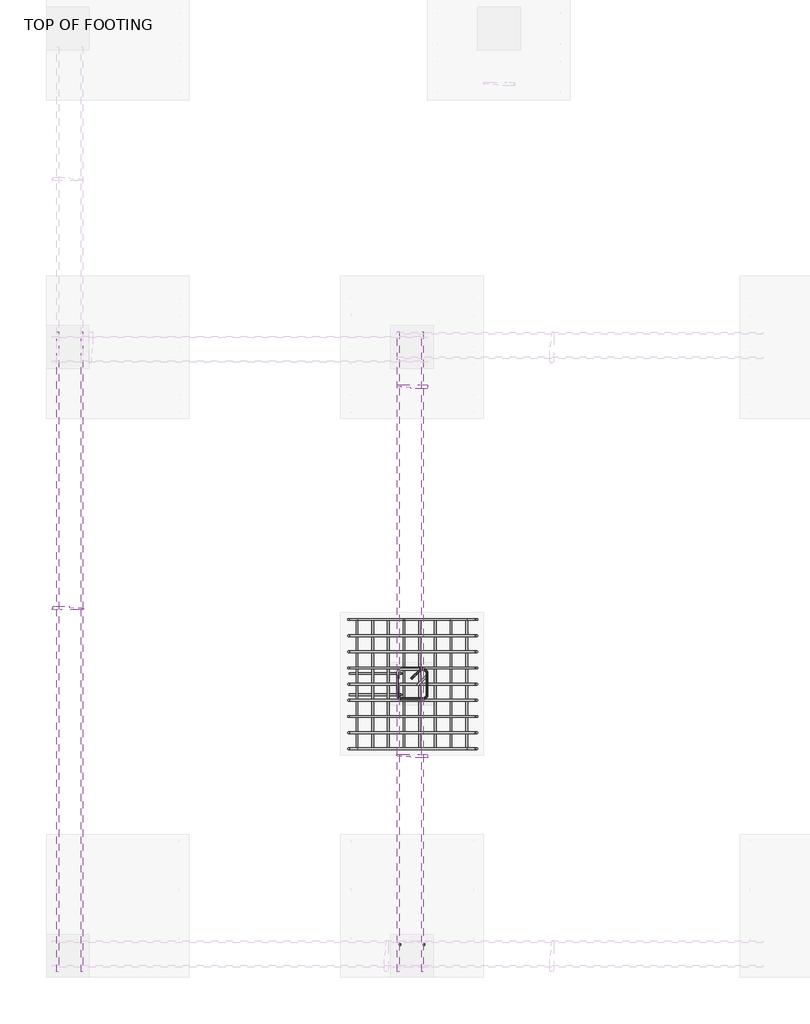
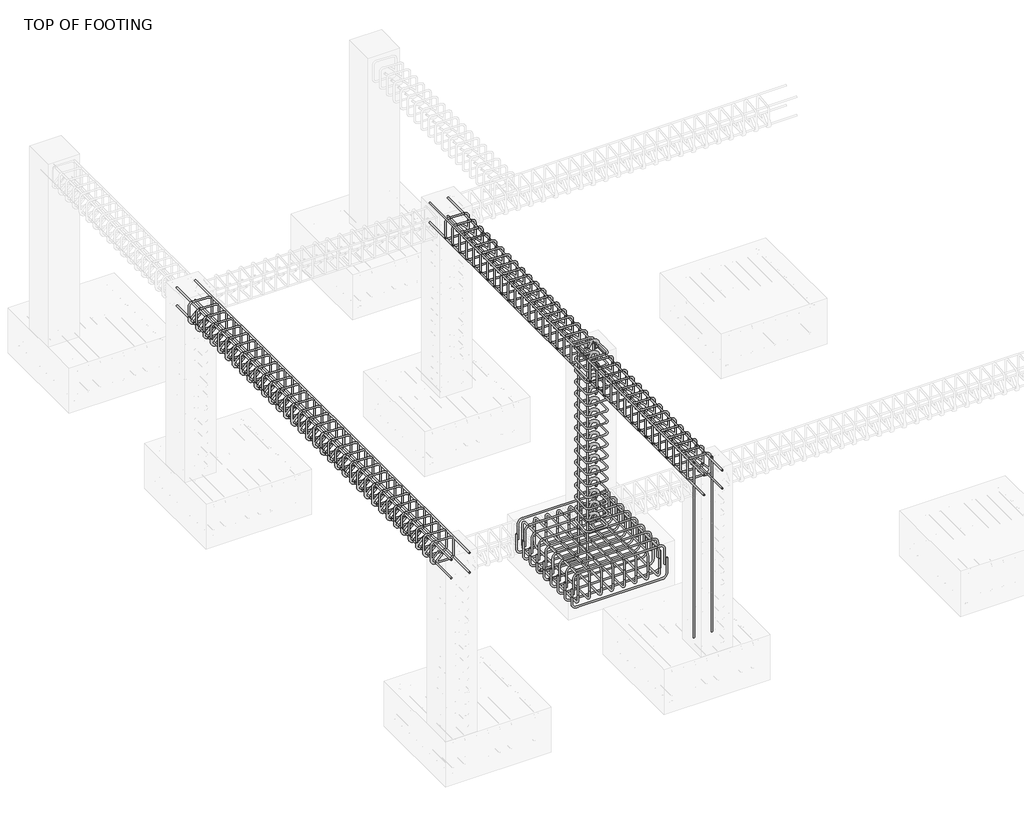
# One storey, part 3 of 10: 16 reinforcing bars.
"""IFC4 building model written with IfcOpenShell, lengths in millimetres."""

from ifc_helpers import new_model, si_unit, point, frame, origin, place, context, project, spatial, polyline, circle_curve, trimmed, segment, composite_curve, source, transform, mapped, element, save
from ifc_brep_helpers import swept_disk

model = new_model("IFC4")

# Units and contexts
model_context = context("Model", 3, world=origin())
ifc_project = project(units=[si_unit("LENGTHUNIT", "METRE", prefix="MILLI")], contexts=[model_context])

# Site, building, storey
site = spatial("IfcSite", under=ifc_project)
building = spatial("IfcBuilding", under=site)
storey = spatial("IfcBuildingStorey", under=building, Name="TOP OF FOOTING", Elevation=-1828.8)

# Reinforcing bars
placement = place(None, origin())
reinforcing_bar_shape = source(origin(), model_context, "Body", "SolidModel", [
    swept_disk(composite_curve([segment(polyline([(-7671.9957678, 10418.4767485, -2013.6880036), (-7671.9957678, 10418.4767485, -2160.9880036)]), True, "CONTINUOUS"), segment(trimmed(circle_curve(frame((-7718.3457678, 10418.4767485, -2160.9880036), z_axis=(0.0, 1.0, 0.0), x_axis=(46.350000000000364, 0.0, 0.0)), 46.35), [point((-7671.9957678, 10418.4767485, -2160.9880036))], [point((-7718.3457678, 10418.4767485, -2207.3380036))], True, "CARTESIAN"), True, "CONTINUOUS"), segment(polyline([(-7718.3457678, 10418.4767485, -2207.3380036), (-8526.0530437, 10418.4767485, -2207.3380036)]), True, "CONTINUOUS"), segment(trimmed(circle_curve(frame((-8526.0530437, 10418.4767485, -2160.9880036), z_axis=(0.0, 1.0, 0.0), x_axis=(0.0, 0.0, -46.34999999999991)), 46.35), [point((-8526.0530437, 10418.4767485, -2207.3380036))], [point((-8572.4030437, 10418.4767485, -2160.9880036))], True, "CARTESIAN"), True, "CONTINUOUS"), segment(polyline([(-8572.4030437, 10418.4767485, -2160.9880036), (-8572.4030437, 10418.4767485, -2013.6880036)]), True, "CONTINUOUS")], self_intersect=False), 6.35),
])
element("IfcReinforcingBar", 1, at=placement, inside=storey, context=model_context, shape_type="MappedRepresentation", body=[
    mapped(reinforcing_bar_shape, transform((0.0, 0.0, 0.0), x_axis=(1.0, 0.0, 0.0), y_axis=(0.0, 1.0, 0.0), z_axis=(0.0, 0.0, 1.0))),
    mapped(reinforcing_bar_shape, transform((0.0, -113.4125, 0.0), x_axis=(1.0, 0.0, 0.0), y_axis=(0.0, 1.0, 0.0), z_axis=(0.0, 0.0, 1.0))),
    mapped(reinforcing_bar_shape, transform((0.0, -226.825, 0.0), x_axis=(1.0, 0.0, 0.0), y_axis=(0.0, 1.0, 0.0), z_axis=(0.0, 0.0, 1.0))),
    mapped(reinforcing_bar_shape, transform((0.0, -340.2375, 0.0), x_axis=(1.0, 0.0, 0.0), y_axis=(0.0, 1.0, 0.0), z_axis=(0.0, 0.0, 1.0))),
    mapped(reinforcing_bar_shape, transform((0.0, -453.65, 0.0), x_axis=(1.0, 0.0, 0.0), y_axis=(0.0, 1.0, 0.0), z_axis=(0.0, 0.0, 1.0))),
    mapped(reinforcing_bar_shape, transform((0.0, -567.0625, 0.0), x_axis=(1.0, 0.0, 0.0), y_axis=(0.0, 1.0, 0.0), z_axis=(0.0, 0.0, 1.0))),
    mapped(reinforcing_bar_shape, transform((0.0, -680.475, 0.0), x_axis=(1.0, 0.0, 0.0), y_axis=(0.0, 1.0, 0.0), z_axis=(0.0, 0.0, 1.0))),
    mapped(reinforcing_bar_shape, transform((0.0, -793.8875, 0.0), x_axis=(1.0, 0.0, 0.0), y_axis=(0.0, 1.0, 0.0), z_axis=(0.0, 0.0, 1.0))),
    mapped(reinforcing_bar_shape, transform((0.0, -907.3, 0.0), x_axis=(1.0, 0.0, 0.0), y_axis=(0.0, 1.0, 0.0), z_axis=(0.0, 0.0, 1.0))),
])
reinforcing_bar_2_shape = source(origin(), model_context, "Body", "SolidModel", [
    swept_disk(composite_curve([segment(polyline([(-8556.1548549, 10418.4767485, -2068.7560969), (-8556.1548549, 10418.4767485, -1921.4560969)]), True, "CONTINUOUS"), segment(trimmed(circle_curve(frame((-8509.8048549, 10418.4767485, -1921.4560969), z_axis=(0.0, 1.0, 0.0), x_axis=(-46.350000000000364, 0.0, 0.0)), 46.35), [point((-8556.1548549, 10418.4767485, -1921.4560969))], [point((-8509.8048549, 10418.4767485, -1875.1060969))], True, "CARTESIAN"), True, "CONTINUOUS"), segment(polyline([(-8509.8048549, 10418.4767485, -1875.1060969), (-7741.4133686, 10418.4767485, -1875.1060969)]), True, "CONTINUOUS"), segment(trimmed(circle_curve(frame((-7741.4133686, 10418.4767485, -1921.4560969), z_axis=(0.0, 1.0, 0.0), x_axis=(0.0, 0.0, 46.34999999999991)), 46.35), [point((-7741.4133686, 10418.4767485, -1875.1060969))], [point((-7695.0633686, 10418.4767485, -1921.4560969))], True, "CARTESIAN"), True, "CONTINUOUS"), segment(polyline([(-7695.0633686, 10418.4767485, -1921.4560969), (-7695.0633686, 10418.4767485, -2068.7560969)]), True, "CONTINUOUS")], self_intersect=False), 6.35),
])
element("IfcReinforcingBar", 2, at=placement, inside=storey, context=model_context, shape_type="MappedRepresentation", body=[
    mapped(reinforcing_bar_2_shape, transform((0.0, 0.0, 0.0), x_axis=(1.0, 0.0, 0.0), y_axis=(0.0, 1.0, 0.0), z_axis=(0.0, 0.0, 1.0))),
    mapped(reinforcing_bar_2_shape, transform((0.0, -113.4125, 0.0), x_axis=(1.0, 0.0, 0.0), y_axis=(0.0, 1.0, 0.0), z_axis=(0.0, 0.0, 1.0))),
    mapped(reinforcing_bar_2_shape, transform((0.0, -226.825, 0.0), x_axis=(1.0, 0.0, 0.0), y_axis=(0.0, 1.0, 0.0), z_axis=(0.0, 0.0, 1.0))),
    mapped(reinforcing_bar_2_shape, transform((0.0, -340.2375, 0.0), x_axis=(1.0, 0.0, 0.0), y_axis=(0.0, 1.0, 0.0), z_axis=(0.0, 0.0, 1.0))),
    mapped(reinforcing_bar_2_shape, transform((0.0, -453.65, 0.0), x_axis=(1.0, 0.0, 0.0), y_axis=(0.0, 1.0, 0.0), z_axis=(0.0, 0.0, 1.0))),
    mapped(reinforcing_bar_2_shape, transform((0.0, -567.0625, 0.0), x_axis=(1.0, 0.0, 0.0), y_axis=(0.0, 1.0, 0.0), z_axis=(0.0, 0.0, 1.0))),
    mapped(reinforcing_bar_2_shape, transform((0.0, -680.475, 0.0), x_axis=(1.0, 0.0, 0.0), y_axis=(0.0, 1.0, 0.0), z_axis=(0.0, 0.0, 1.0))),
    mapped(reinforcing_bar_2_shape, transform((0.0, -793.8875, 0.0), x_axis=(1.0, 0.0, 0.0), y_axis=(0.0, 1.0, 0.0), z_axis=(0.0, 0.0, 1.0))),
    mapped(reinforcing_bar_2_shape, transform((0.0, -907.3, 0.0), x_axis=(1.0, 0.0, 0.0), y_axis=(0.0, 1.0, 0.0), z_axis=(0.0, 0.0, 1.0))),
])
reinforcing_bar_3_shape = source(origin(), model_context, "Body", "SolidModel", [
    swept_disk(composite_curve([segment(polyline([(-7744.2682872, 10418.4767485, -2087.4821199), (-7744.2682872, 10418.4767485, -1940.1821199)]), True, "CONTINUOUS"), segment(trimmed(circle_curve(frame((-7744.2682872, 10372.1267485, -1940.1821199), z_axis=(1.0, 0.0, 0.0), x_axis=(0.0, 46.349999999998545, 0.0)), 46.35), [point((-7744.2682872, 10418.4767485, -1940.1821199))], [point((-7744.2682872, 10372.1267485, -1893.8321199))], True, "CARTESIAN"), True, "CONTINUOUS"), segment(polyline([(-7744.2682872, 10372.1267485, -1893.8321199), (-7744.2682872, 9557.5267485, -1893.8321199)]), True, "CONTINUOUS"), segment(trimmed(circle_curve(frame((-7744.2682872, 9557.5267485, -1940.1821199), z_axis=(1.0, 0.0, 0.0), x_axis=(0.0, 0.0, 46.350000000000136)), 46.35), [point((-7744.2682872, 9557.5267485, -1893.8321199))], [point((-7744.2682872, 9511.1767485, -1940.1821199))], True, "CARTESIAN"), True, "CONTINUOUS"), segment(polyline([(-7744.2682872, 9511.1767485, -1940.1821199), (-7744.2682872, 9511.1767485, -2087.4821199)]), True, "CONTINUOUS")], self_intersect=False), 6.35),
])
element("IfcReinforcingBar", 3, at=placement, inside=storey, context=model_context, shape_type="MappedRepresentation", body=[
    mapped(reinforcing_bar_3_shape, transform((0.0, 0.0, 0.0), x_axis=(1.0, 0.0, 0.0), y_axis=(0.0, 1.0, 0.0), z_axis=(0.0, 0.0, 1.0))),
    mapped(reinforcing_bar_3_shape, transform((-109.824938, 0.0, 0.0), x_axis=(1.0, 0.0, 0.0), y_axis=(0.0, 1.0, 0.0), z_axis=(0.0, 0.0, 1.0))),
    mapped(reinforcing_bar_3_shape, transform((-219.649876, 0.0, 0.0), x_axis=(1.0, 0.0, 0.0), y_axis=(0.0, 1.0, 0.0), z_axis=(0.0, 0.0, 1.0))),
    mapped(reinforcing_bar_3_shape, transform((-329.474814, 0.0, 0.0), x_axis=(1.0, 0.0, 0.0), y_axis=(0.0, 1.0, 0.0), z_axis=(0.0, 0.0, 1.0))),
    mapped(reinforcing_bar_3_shape, transform((-439.299752, 0.0, 0.0), x_axis=(1.0, 0.0, 0.0), y_axis=(0.0, 1.0, 0.0), z_axis=(0.0, 0.0, 1.0))),
    mapped(reinforcing_bar_3_shape, transform((-549.12469, 0.0, 0.0), x_axis=(1.0, 0.0, 0.0), y_axis=(0.0, 1.0, 0.0), z_axis=(0.0, 0.0, 1.0))),
    mapped(reinforcing_bar_3_shape, transform((-658.949628, 0.0, 0.0), x_axis=(1.0, 0.0, 0.0), y_axis=(0.0, 1.0, 0.0), z_axis=(0.0, 0.0, 1.0))),
    mapped(reinforcing_bar_3_shape, transform((-768.774566, 0.0, 0.0), x_axis=(1.0, 0.0, 0.0), y_axis=(0.0, 1.0, 0.0), z_axis=(0.0, 0.0, 1.0))),
])
reinforcing_bar_4_shape = source(origin(), model_context, "Body", "SolidModel", [
    swept_disk(composite_curve([segment(polyline([(-8513.0428532, 10418.4767485, -1990.1985611), (-8513.0428532, 10418.4767485, -2137.4985611)]), True, "CONTINUOUS"), segment(trimmed(circle_curve(frame((-8513.0428532, 10372.1267485, -2137.4985611), z_axis=(-1.0, 0.0, 0.0), x_axis=(0.0, 46.349999999998545, 0.0)), 46.35), [point((-8513.0428532, 10418.4767485, -2137.4985611))], [point((-8513.0428532, 10372.1267485, -2183.8485611))], True, "CARTESIAN"), True, "CONTINUOUS"), segment(polyline([(-8513.0428532, 10372.1267485, -2183.8485611), (-8513.0428532, 9557.5267485, -2183.8485611)]), True, "CONTINUOUS"), segment(trimmed(circle_curve(frame((-8513.0428532, 9557.5267485, -2137.4985611), z_axis=(-1.0, 0.0, 0.0), x_axis=(0.0, 0.0, -46.34999999999991)), 46.35), [point((-8513.0428532, 9557.5267485, -2183.8485611))], [point((-8513.0428532, 9511.1767485, -2137.4985611))], True, "CARTESIAN"), True, "CONTINUOUS"), segment(polyline([(-8513.0428532, 9511.1767485, -2137.4985611), (-8513.0428532, 9511.1767485, -1990.1985611)]), True, "CONTINUOUS")], self_intersect=False), 6.35),
])
element("IfcReinforcingBar", 4, at=placement, inside=storey, context=model_context, shape_type="MappedRepresentation", body=[
    mapped(reinforcing_bar_4_shape, transform((0.0, 0.0, 0.0), x_axis=(1.0, 0.0, 0.0), y_axis=(0.0, 1.0, 0.0), z_axis=(0.0, 0.0, 1.0))),
    mapped(reinforcing_bar_4_shape, transform((109.824938, 0.0, 0.0), x_axis=(1.0, 0.0, 0.0), y_axis=(0.0, 1.0, 0.0), z_axis=(0.0, 0.0, 1.0))),
    mapped(reinforcing_bar_4_shape, transform((219.649876, 0.0, 0.0), x_axis=(1.0, 0.0, 0.0), y_axis=(0.0, 1.0, 0.0), z_axis=(0.0, 0.0, 1.0))),
    mapped(reinforcing_bar_4_shape, transform((329.474814, 0.0, 0.0), x_axis=(1.0, 0.0, 0.0), y_axis=(0.0, 1.0, 0.0), z_axis=(0.0, 0.0, 1.0))),
    mapped(reinforcing_bar_4_shape, transform((439.299752, 0.0, 0.0), x_axis=(1.0, 0.0, 0.0), y_axis=(0.0, 1.0, 0.0), z_axis=(0.0, 0.0, 1.0))),
    mapped(reinforcing_bar_4_shape, transform((549.12469, 0.0, 0.0), x_axis=(1.0, 0.0, 0.0), y_axis=(0.0, 1.0, 0.0), z_axis=(0.0, 0.0, 1.0))),
    mapped(reinforcing_bar_4_shape, transform((658.949628, 0.0, 0.0), x_axis=(1.0, 0.0, 0.0), y_axis=(0.0, 1.0, 0.0), z_axis=(0.0, 0.0, 1.0))),
    mapped(reinforcing_bar_4_shape, transform((768.774566, 0.0, 0.0), x_axis=(1.0, 0.0, 0.0), y_axis=(0.0, 1.0, 0.0), z_axis=(0.0, 0.0, 1.0))),
])
reinforcing_bar_5_shape = source(origin(), model_context, "Body", "SolidModel", [
    swept_disk(composite_curve([segment(polyline([(-8131.2571284, 10003.5509831, -57.3273613), (-8075.5135654, 10059.2945461, -57.3273613)]), True, "CONTINUOUS"), segment(trimmed(circle_curve(frame((-8053.3457678, 10037.1267485, -57.3273613), z_axis=(0.0, 0.0, -1.0), x_axis=(-22.167797599999176, 22.167797599999176, 0.0)), 31.35), [point((-8075.5135654, 10059.2945461, -57.3273613))], [point((-8021.9957678, 10037.1267485, -57.3273613))], True, "CARTESIAN"), True, "CONTINUOUS"), segment(polyline([(-8021.9957678, 10037.1267485, -57.3273613), (-8021.9957678, 9892.5267485, -57.3273613)]), True, "CONTINUOUS"), segment(trimmed(circle_curve(frame((-8053.3457678, 9892.5267485, -57.3273613), z_axis=(0.0, 0.0, -1.0), x_axis=(31.350000000000364, 0.0, 0.0)), 31.35), [point((-8021.9957678, 9892.5267485, -57.3273613))], [point((-8053.3457678, 9861.1767485, -57.3273613))], True, "CARTESIAN"), True, "CONTINUOUS"), segment(polyline([(-8053.3457678, 9861.1767485, -57.3273613), (-8197.9457678, 9861.1767485, -57.3273613)]), True, "CONTINUOUS"), segment(trimmed(circle_curve(frame((-8197.9457678, 9892.4680812, -55.4103332), z_axis=(0.0, 0.06114922175001322, -0.9981286353368326), x_axis=(0.0, -31.291332700000567, -1.9170281000000031)), 31.35), [point((-8197.9457678, 9861.1767485, -57.3273613))], [point((-8229.2957678, 9892.4680812, -55.4103332))], True, "CARTESIAN"), True, "CONTINUOUS"), segment(polyline([(-8229.2957678, 9892.4680812, -55.4103332), (-8229.2957678, 10037.1854158, -46.5443894)]), True, "CONTINUOUS"), segment(trimmed(circle_curve(frame((-8197.9457678, 10037.1854158, -46.5443894), z_axis=(0.0, 0.06114922175001322, -0.9981286353368326), x_axis=(-31.350000000000364, 0.0, 0.0)), 31.35), [point((-8229.2957678, 10037.1854158, -46.5443894))], [point((-8197.9457678, 10068.4767485, -44.6273613))], True, "CARTESIAN"), True, "CONTINUOUS"), segment(polyline([(-8197.9457678, 10068.4767485, -44.6273613), (-8053.3457678, 10068.4767485, -44.6273613)]), True, "CONTINUOUS"), segment(trimmed(circle_curve(frame((-8053.3457678, 10037.1267485, -44.6273613), z_axis=(0.0, 0.0, -1.0), x_axis=(0.0, 31.349999999998545, 0.0)), 31.35), [point((-8053.3457678, 10068.4767485, -44.6273613))], [point((-8031.1779702, 10014.9589509, -44.6273613))], True, "CARTESIAN"), True, "CONTINUOUS"), segment(polyline([(-8031.1779702, 10014.9589509, -44.6273613), (-8086.9215332, 9959.2153879, -44.6273613)]), True, "CONTINUOUS")], self_intersect=False), 6.35),
])
element("IfcReinforcingBar", 5, at=placement, inside=storey, context=model_context, shape_type="MappedRepresentation", body=[
    mapped(reinforcing_bar_5_shape, transform((0.0, 0.0, 0.0), x_axis=(1.0, 0.0, 0.0), y_axis=(0.0, 1.0, 0.0), z_axis=(0.0, 0.0, 1.0))),
    mapped(reinforcing_bar_5_shape, transform((0.0, 0.0, -115.0081759), x_axis=(1.0, 0.0, 0.0), y_axis=(0.0, 1.0, 0.0), z_axis=(0.0, 0.0, 1.0))),
    mapped(reinforcing_bar_5_shape, transform((0.0, 0.0, -230.0163518), x_axis=(1.0, 0.0, 0.0), y_axis=(0.0, 1.0, 0.0), z_axis=(0.0, 0.0, 1.0))),
    mapped(reinforcing_bar_5_shape, transform((0.0, 0.0, -345.0245277), x_axis=(1.0, 0.0, 0.0), y_axis=(0.0, 1.0, 0.0), z_axis=(0.0, 0.0, 1.0))),
    mapped(reinforcing_bar_5_shape, transform((0.0, 0.0, -460.0327037), x_axis=(1.0, 0.0, 0.0), y_axis=(0.0, 1.0, 0.0), z_axis=(0.0, 0.0, 1.0))),
    mapped(reinforcing_bar_5_shape, transform((0.0, 0.0, -575.0408796), x_axis=(1.0, 0.0, 0.0), y_axis=(0.0, 1.0, 0.0), z_axis=(0.0, 0.0, 1.0))),
    mapped(reinforcing_bar_5_shape, transform((0.0, 0.0, -690.0490555), x_axis=(1.0, 0.0, 0.0), y_axis=(0.0, 1.0, 0.0), z_axis=(0.0, 0.0, 1.0))),
    mapped(reinforcing_bar_5_shape, transform((0.0, 0.0, -805.0572314), x_axis=(1.0, 0.0, 0.0), y_axis=(0.0, 1.0, 0.0), z_axis=(0.0, 0.0, 1.0))),
    mapped(reinforcing_bar_5_shape, transform((0.0, 0.0, -920.0654073), x_axis=(1.0, 0.0, 0.0), y_axis=(0.0, 1.0, 0.0), z_axis=(0.0, 0.0, 1.0))),
    mapped(reinforcing_bar_5_shape, transform((0.0, 0.0, -1035.0735832), x_axis=(1.0, 0.0, 0.0), y_axis=(0.0, 1.0, 0.0), z_axis=(0.0, 0.0, 1.0))),
    mapped(reinforcing_bar_5_shape, transform((0.0, 0.0, -1150.0817591), x_axis=(1.0, 0.0, 0.0), y_axis=(0.0, 1.0, 0.0), z_axis=(0.0, 0.0, 1.0))),
    mapped(reinforcing_bar_5_shape, transform((0.0, 0.0, -1265.0899351), x_axis=(1.0, 0.0, 0.0), y_axis=(0.0, 1.0, 0.0), z_axis=(0.0, 0.0, 1.0))),
    mapped(reinforcing_bar_5_shape, transform((0.0, 0.0, -1380.098111), x_axis=(1.0, 0.0, 0.0), y_axis=(0.0, 1.0, 0.0), z_axis=(0.0, 0.0, 1.0))),
    mapped(reinforcing_bar_5_shape, transform((0.0, 0.0, -1495.1062869), x_axis=(1.0, 0.0, 0.0), y_axis=(0.0, 1.0, 0.0), z_axis=(0.0, 0.0, 1.0))),
    mapped(reinforcing_bar_5_shape, transform((0.0, 0.0, -1610.1144628), x_axis=(1.0, 0.0, 0.0), y_axis=(0.0, 1.0, 0.0), z_axis=(0.0, 0.0, 1.0))),
    mapped(reinforcing_bar_5_shape, transform((0.0, 0.0, -1725.1226387), x_axis=(1.0, 0.0, 0.0), y_axis=(0.0, 1.0, 0.0), z_axis=(0.0, 0.0, 1.0))),
])
reinforcing_bar_6_shape = source(origin(), model_context, "Body", "SolidModel", [
    swept_disk(composite_curve([segment(polyline([(-8205.4457678, 10039.3167668, -40.0), (-8205.4457678, 10039.3167668, -2102.45)]), True, "CONTINUOUS"), segment(trimmed(circle_curve(frame((-8251.7957678, 10039.3167668, -2102.45), z_axis=(0.0, 1.0, 0.0), x_axis=(46.350000000000364, 0.0, 0.0)), 46.35), [point((-8205.4457678, 10039.3167668, -2102.45))], [point((-8251.7957678, 10039.3167668, -2148.8))], True, "CARTESIAN"), True, "CONTINUOUS"), segment(polyline([(-8251.7957678, 10039.3167668, -2148.8), (-8566.0530437, 10039.3167668, -2148.8)]), True, "CONTINUOUS")], self_intersect=False), 6.35),
])
element("IfcReinforcingBar", 6, at=placement, inside=storey, context=model_context, shape_type="MappedRepresentation", body=[
    mapped(reinforcing_bar_6_shape, transform((0.0, 0.0, 0.0), x_axis=(1.0, 0.0, 0.0), y_axis=(0.0, 1.0, 0.0), z_axis=(0.0, 0.0, 1.0))),
    mapped(reinforcing_bar_6_shape, transform((0.0, -149.7926021, 0.0), x_axis=(1.0, 0.0, 0.0), y_axis=(0.0, 1.0, 0.0), z_axis=(0.0, 0.0, 1.0))),
])
reinforcing_bar_7_shape = source(origin(), model_context, "Body", "SolidModel", [
    swept_disk(composite_curve([segment(polyline([(-8042.7163335, 8137.2267485, -1788.8), (-8042.7163335, 8137.2267485, -40.0)]), True, "CONTINUOUS")], self_intersect=False), 6.35),
])
element("IfcReinforcingBar", 7, at=placement, inside=storey, context=model_context, shape_type="MappedRepresentation", body=[
    mapped(reinforcing_bar_7_shape, transform((0.0, 0.0, 0.0), x_axis=(1.0, 0.0, 0.0), y_axis=(0.0, 1.0, 0.0), z_axis=(0.0, 0.0, 1.0))),
    mapped(reinforcing_bar_7_shape, transform((-168.8572682, 0.0, 0.0), x_axis=(1.0, 0.0, 0.0), y_axis=(0.0, 1.0, 0.0), z_axis=(0.0, 0.0, 1.0))),
])
reinforcing_bar_8_shape = source(origin(), model_context, "Body", "SolidModel", [
    swept_disk(composite_curve([segment(polyline([(-8086.9215332, 10121.1767485, -144.3886395), (-8031.1779702, 10121.1767485, -200.1322024)]), True, "CONTINUOUS"), segment(trimmed(circle_curve(frame((-8053.3457678, 10121.1767485, -222.3), z_axis=(0.0, 1.0, 0.0), x_axis=(22.167797600000085, 0.0, 22.1677976)), 31.35), [point((-8031.1779702, 10121.1767485, -200.1322024))], [point((-8053.3457678, 10121.1767485, -253.65))], True, "CARTESIAN"), True, "CONTINUOUS"), segment(polyline([(-8053.3457678, 10121.1767485, -253.65), (-8197.9457678, 10121.1767485, -253.65)]), True, "CONTINUOUS"), segment(trimmed(circle_curve(frame((-8197.9457678, 10121.1767485, -222.3), z_axis=(0.0, 1.0, 0.0), x_axis=(0.0, 0.0, -31.349999999999994)), 31.35), [point((-8197.9457678, 10121.1767485, -253.65))], [point((-8229.2957678, 10121.1767485, -222.3))], True, "CARTESIAN"), True, "CONTINUOUS"), segment(polyline([(-8229.2957678, 10121.1767485, -222.3), (-8229.2957678, 10121.1767485, -77.7)]), True, "CONTINUOUS"), segment(trimmed(circle_curve(frame((-8198.0044351, 10119.2597204, -77.7), z_axis=(0.06114922175001232, 0.9981286353368327, 0.0), x_axis=(-31.291332700000567, 1.917028100000607, 0.0)), 31.35), [point((-8229.2957678, 10121.1767485, -77.7))], [point((-8198.0044351, 10119.2597204, -46.35))], True, "CARTESIAN"), True, "CONTINUOUS"), segment(polyline([(-8198.0044351, 10119.2597204, -46.35), (-8053.2871006, 10110.3937766, -46.35)]), True, "CONTINUOUS"), segment(trimmed(circle_curve(frame((-8053.2871006, 10110.3937766, -77.7), z_axis=(0.06114922175001232, 0.9981286353368327, 0.0), x_axis=(0.0, 0.0, 31.35)), 31.35), [point((-8053.2871006, 10110.3937766, -46.35))], [point((-8021.9957678, 10108.4767485, -77.7))], True, "CARTESIAN"), True, "CONTINUOUS"), segment(polyline([(-8021.9957678, 10108.4767485, -77.7), (-8021.9957678, 10108.4767485, -222.3)]), True, "CONTINUOUS"), segment(trimmed(circle_curve(frame((-8053.3457678, 10108.4767485, -222.3), z_axis=(0.0, 1.0, 0.0), x_axis=(31.350000000000364, 0.0, 0.0)), 31.35), [point((-8021.9957678, 10108.4767485, -222.3))], [point((-8075.5135654, 10108.4767485, -244.4677976))], True, "CARTESIAN"), True, "CONTINUOUS"), segment(polyline([(-8075.5135654, 10108.4767485, -244.4677976), (-8131.2571284, 10108.4767485, -188.7242346)]), True, "CONTINUOUS")], self_intersect=False), 6.35),
])
element("IfcReinforcingBar", 8, at=placement, inside=storey, context=model_context, shape_type="MappedRepresentation", body=[
    mapped(reinforcing_bar_8_shape, transform((0.0, 0.0, 0.0), x_axis=(1.0, 0.0, 0.0), y_axis=(0.0, 1.0, 0.0), z_axis=(0.0, 0.0, 1.0))),
    mapped(reinforcing_bar_8_shape, transform((0.0, 113.8611111, 0.0), x_axis=(1.0, 0.0, 0.0), y_axis=(0.0, 1.0, 0.0), z_axis=(0.0, 0.0, 1.0))),
    mapped(reinforcing_bar_8_shape, transform((0.0, 227.7222222, 0.0), x_axis=(1.0, 0.0, 0.0), y_axis=(0.0, 1.0, 0.0), z_axis=(0.0, 0.0, 1.0))),
    mapped(reinforcing_bar_8_shape, transform((0.0, 341.5833333, 0.0), x_axis=(1.0, 0.0, 0.0), y_axis=(0.0, 1.0, 0.0), z_axis=(0.0, 0.0, 1.0))),
    mapped(reinforcing_bar_8_shape, transform((0.0, 455.4444444, 0.0), x_axis=(1.0, 0.0, 0.0), y_axis=(0.0, 1.0, 0.0), z_axis=(0.0, 0.0, 1.0))),
    mapped(reinforcing_bar_8_shape, transform((0.0, 569.3055556, 0.0), x_axis=(1.0, 0.0, 0.0), y_axis=(0.0, 1.0, 0.0), z_axis=(0.0, 0.0, 1.0))),
    mapped(reinforcing_bar_8_shape, transform((0.0, 683.1666667, 0.0), x_axis=(1.0, 0.0, 0.0), y_axis=(0.0, 1.0, 0.0), z_axis=(0.0, 0.0, 1.0))),
    mapped(reinforcing_bar_8_shape, transform((0.0, 797.0277778, 0.0), x_axis=(1.0, 0.0, 0.0), y_axis=(0.0, 1.0, 0.0), z_axis=(0.0, 0.0, 1.0))),
    mapped(reinforcing_bar_8_shape, transform((0.0, 910.8888889, 0.0), x_axis=(1.0, 0.0, 0.0), y_axis=(0.0, 1.0, 0.0), z_axis=(0.0, 0.0, 1.0))),
    mapped(reinforcing_bar_8_shape, transform((0.0, 1024.75, 0.0), x_axis=(1.0, 0.0, 0.0), y_axis=(0.0, 1.0, 0.0), z_axis=(0.0, 0.0, 1.0))),
    mapped(reinforcing_bar_8_shape, transform((0.0, 1138.6111111, 0.0), x_axis=(1.0, 0.0, 0.0), y_axis=(0.0, 1.0, 0.0), z_axis=(0.0, 0.0, 1.0))),
    mapped(reinforcing_bar_8_shape, transform((0.0, 1252.4722222, 0.0), x_axis=(1.0, 0.0, 0.0), y_axis=(0.0, 1.0, 0.0), z_axis=(0.0, 0.0, 1.0))),
    mapped(reinforcing_bar_8_shape, transform((0.0, 1366.3333333, 0.0), x_axis=(1.0, 0.0, 0.0), y_axis=(0.0, 1.0, 0.0), z_axis=(0.0, 0.0, 1.0))),
    mapped(reinforcing_bar_8_shape, transform((0.0, 1480.1944444, 0.0), x_axis=(1.0, 0.0, 0.0), y_axis=(0.0, 1.0, 0.0), z_axis=(0.0, 0.0, 1.0))),
    mapped(reinforcing_bar_8_shape, transform((0.0, 1594.0555556, 0.0), x_axis=(1.0, 0.0, 0.0), y_axis=(0.0, 1.0, 0.0), z_axis=(0.0, 0.0, 1.0))),
    mapped(reinforcing_bar_8_shape, transform((0.0, 1707.9166667, 0.0), x_axis=(1.0, 0.0, 0.0), y_axis=(0.0, 1.0, 0.0), z_axis=(0.0, 0.0, 1.0))),
    mapped(reinforcing_bar_8_shape, transform((0.0, 1821.7777778, 0.0), x_axis=(1.0, 0.0, 0.0), y_axis=(0.0, 1.0, 0.0), z_axis=(0.0, 0.0, 1.0))),
    mapped(reinforcing_bar_8_shape, transform((0.0, 1935.6388889, 0.0), x_axis=(1.0, 0.0, 0.0), y_axis=(0.0, 1.0, 0.0), z_axis=(0.0, 0.0, 1.0))),
    mapped(reinforcing_bar_8_shape, transform((0.0, 2049.5, 0.0), x_axis=(1.0, 0.0, 0.0), y_axis=(0.0, 1.0, 0.0), z_axis=(0.0, 0.0, 1.0))),
])
reinforcing_bar_9_shape = source(origin(), model_context, "Body", "SolidModel", [
    swept_disk(composite_curve([segment(polyline([(-8053.3457678, 9854.8267485, -240.95), (-8053.3457678, 12437.0267485, -240.95)]), True, "CONTINUOUS")], self_intersect=False), 6.35),
])
element("IfcReinforcingBar", 9, at=placement, inside=storey, context=model_context, shape_type="MappedRepresentation", body=[
    mapped(reinforcing_bar_9_shape, transform((0.0, 0.0, 0.0), x_axis=(1.0, 0.0, 0.0), y_axis=(0.0, 1.0, 0.0), z_axis=(0.0, 0.0, 1.0))),
    mapped(reinforcing_bar_9_shape, transform((0.0, 0.0, 181.9), x_axis=(1.0, 0.0, 0.0), y_axis=(0.0, 1.0, 0.0), z_axis=(0.0, 0.0, 1.0))),
])
reinforcing_bar_10_shape = source(origin(), model_context, "Body", "SolidModel", [
    swept_disk(composite_curve([segment(polyline([(-8224.9457678, 9854.8267485, -245.5918309), (-8224.9457678, 12437.0267485, -245.5918309)]), True, "CONTINUOUS")], self_intersect=False), 6.35),
])
element("IfcReinforcingBar", 10, at=placement, inside=storey, context=model_context, shape_type="MappedRepresentation", body=[
    mapped(reinforcing_bar_10_shape, transform((0.0, 0.0, 0.0), x_axis=(1.0, 0.0, 0.0), y_axis=(0.0, 1.0, 0.0), z_axis=(0.0, 0.0, 1.0))),
    mapped(reinforcing_bar_10_shape, transform((0.0, 0.0, 197.4676357), x_axis=(1.0, 0.0, 0.0), y_axis=(0.0, 1.0, 0.0), z_axis=(0.0, 0.0, 1.0))),
])
reinforcing_bar_11_shape = source(origin(), model_context, "Body", "SolidModel", [
    swept_disk(composite_curve([segment(polyline([(-10579.7700025, 12170.6767485, -144.3886395), (-10635.5135654, 12170.6767485, -200.1322024)]), True, "CONTINUOUS"), segment(trimmed(circle_curve(frame((-10613.3457678, 12170.6767485, -222.3), z_axis=(0.0, -1.0, 0.0), x_axis=(-22.167797600000995, 0.0, 22.1677976)), 31.35), [point((-10635.5135654, 12170.6767485, -200.1322024))], [point((-10613.3457678, 12170.6767485, -253.65))], True, "CARTESIAN"), True, "CONTINUOUS"), segment(polyline([(-10613.3457678, 12170.6767485, -253.65), (-10468.7457678, 12170.6767485, -253.65)]), True, "CONTINUOUS"), segment(trimmed(circle_curve(frame((-10468.7457678, 12170.6767485, -222.3), z_axis=(0.0, -1.0, 0.0), x_axis=(0.0, 0.0, -31.349999999999994)), 31.35), [point((-10468.7457678, 12170.6767485, -253.65))], [point((-10437.3957678, 12170.6767485, -222.3))], True, "CARTESIAN"), True, "CONTINUOUS"), segment(polyline([(-10437.3957678, 12170.6767485, -222.3), (-10437.3957678, 12170.6767485, -77.7)]), True, "CONTINUOUS"), segment(trimmed(circle_curve(frame((-10468.6871006, 12172.5937766, -77.7), z_axis=(-0.06114922175001206, -0.9981286353368327, 0.0), x_axis=(31.29133279999951, -1.917028100000607, 0.0)), 31.35), [point((-10437.3957678, 12170.6767485, -77.7))], [point((-10468.6871006, 12172.5937766, -46.35))], True, "CARTESIAN"), True, "CONTINUOUS"), segment(polyline([(-10468.6871006, 12172.5937766, -46.35), (-10613.4044351, 12181.4597204, -46.35)]), True, "CONTINUOUS"), segment(trimmed(circle_curve(frame((-10613.4044351, 12181.4597204, -77.7), z_axis=(-0.06114922175001206, -0.9981286353368327, 0.0), x_axis=(0.0, 0.0, 31.35)), 31.35), [point((-10613.4044351, 12181.4597204, -46.35))], [point((-10644.6957678, 12183.3767485, -77.7))], True, "CARTESIAN"), True, "CONTINUOUS"), segment(polyline([(-10644.6957678, 12183.3767485, -77.7), (-10644.6957678, 12183.3767485, -222.3)]), True, "CONTINUOUS"), segment(trimmed(circle_curve(frame((-10613.3457678, 12183.3767485, -222.3), z_axis=(0.0, -1.0, 0.0), x_axis=(-31.350000000000364, 0.0, 0.0)), 31.35), [point((-10644.6957678, 12183.3767485, -222.3))], [point((-10591.1779702, 12183.3767485, -244.4677976))], True, "CARTESIAN"), True, "CONTINUOUS"), segment(polyline([(-10591.1779702, 12183.3767485, -244.4677976), (-10535.4344073, 12183.3767485, -188.7242346)]), True, "CONTINUOUS")], self_intersect=False), 6.35),
])
element("IfcReinforcingBar", 11, at=placement, inside=storey, context=model_context, shape_type="MappedRepresentation", body=[
    mapped(reinforcing_bar_11_shape, transform((0.0, 0.0, 0.0), x_axis=(1.0, 0.0, 0.0), y_axis=(0.0, 1.0, 0.0), z_axis=(0.0, 0.0, 1.0))),
    mapped(reinforcing_bar_11_shape, transform((0.0, -119.9060606, 0.0), x_axis=(1.0, 0.0, 0.0), y_axis=(0.0, 1.0, 0.0), z_axis=(0.0, 0.0, 1.0))),
    mapped(reinforcing_bar_11_shape, transform((0.0, -239.8121212, 0.0), x_axis=(1.0, 0.0, 0.0), y_axis=(0.0, 1.0, 0.0), z_axis=(0.0, 0.0, 1.0))),
    mapped(reinforcing_bar_11_shape, transform((0.0, -359.7181818, 0.0), x_axis=(1.0, 0.0, 0.0), y_axis=(0.0, 1.0, 0.0), z_axis=(0.0, 0.0, 1.0))),
    mapped(reinforcing_bar_11_shape, transform((0.0, -479.6242424, 0.0), x_axis=(1.0, 0.0, 0.0), y_axis=(0.0, 1.0, 0.0), z_axis=(0.0, 0.0, 1.0))),
    mapped(reinforcing_bar_11_shape, transform((0.0, -599.530303, 0.0), x_axis=(1.0, 0.0, 0.0), y_axis=(0.0, 1.0, 0.0), z_axis=(0.0, 0.0, 1.0))),
    mapped(reinforcing_bar_11_shape, transform((0.0, -719.4363636, 0.0), x_axis=(1.0, 0.0, 0.0), y_axis=(0.0, 1.0, 0.0), z_axis=(0.0, 0.0, 1.0))),
    mapped(reinforcing_bar_11_shape, transform((0.0, -839.3424242, 0.0), x_axis=(1.0, 0.0, 0.0), y_axis=(0.0, 1.0, 0.0), z_axis=(0.0, 0.0, 1.0))),
    mapped(reinforcing_bar_11_shape, transform((0.0, -959.2484848, 0.0), x_axis=(1.0, 0.0, 0.0), y_axis=(0.0, 1.0, 0.0), z_axis=(0.0, 0.0, 1.0))),
    mapped(reinforcing_bar_11_shape, transform((0.0, -1079.1545455, 0.0), x_axis=(1.0, 0.0, 0.0), y_axis=(0.0, 1.0, 0.0), z_axis=(0.0, 0.0, 1.0))),
    mapped(reinforcing_bar_11_shape, transform((0.0, -1199.0606061, 0.0), x_axis=(1.0, 0.0, 0.0), y_axis=(0.0, 1.0, 0.0), z_axis=(0.0, 0.0, 1.0))),
    mapped(reinforcing_bar_11_shape, transform((0.0, -1318.9666667, 0.0), x_axis=(1.0, 0.0, 0.0), y_axis=(0.0, 1.0, 0.0), z_axis=(0.0, 0.0, 1.0))),
    mapped(reinforcing_bar_11_shape, transform((0.0, -1438.8727273, 0.0), x_axis=(1.0, 0.0, 0.0), y_axis=(0.0, 1.0, 0.0), z_axis=(0.0, 0.0, 1.0))),
    mapped(reinforcing_bar_11_shape, transform((0.0, -1558.7787879, 0.0), x_axis=(1.0, 0.0, 0.0), y_axis=(0.0, 1.0, 0.0), z_axis=(0.0, 0.0, 1.0))),
    mapped(reinforcing_bar_11_shape, transform((0.0, -1678.6848485, 0.0), x_axis=(1.0, 0.0, 0.0), y_axis=(0.0, 1.0, 0.0), z_axis=(0.0, 0.0, 1.0))),
    mapped(reinforcing_bar_11_shape, transform((0.0, -1798.5909091, 0.0), x_axis=(1.0, 0.0, 0.0), y_axis=(0.0, 1.0, 0.0), z_axis=(0.0, 0.0, 1.0))),
    mapped(reinforcing_bar_11_shape, transform((0.0, -1918.4969697, 0.0), x_axis=(1.0, 0.0, 0.0), y_axis=(0.0, 1.0, 0.0), z_axis=(0.0, 0.0, 1.0))),
    mapped(reinforcing_bar_11_shape, transform((0.0, -2038.4030303, 0.0), x_axis=(1.0, 0.0, 0.0), y_axis=(0.0, 1.0, 0.0), z_axis=(0.0, 0.0, 1.0))),
    mapped(reinforcing_bar_11_shape, transform((0.0, -2158.3090909, 0.0), x_axis=(1.0, 0.0, 0.0), y_axis=(0.0, 1.0, 0.0), z_axis=(0.0, 0.0, 1.0))),
    mapped(reinforcing_bar_11_shape, transform((0.0, -2278.2151515, 0.0), x_axis=(1.0, 0.0, 0.0), y_axis=(0.0, 1.0, 0.0), z_axis=(0.0, 0.0, 1.0))),
    mapped(reinforcing_bar_11_shape, transform((0.0, -2398.1212121, 0.0), x_axis=(1.0, 0.0, 0.0), y_axis=(0.0, 1.0, 0.0), z_axis=(0.0, 0.0, 1.0))),
    mapped(reinforcing_bar_11_shape, transform((0.0, -2518.0272727, 0.0), x_axis=(1.0, 0.0, 0.0), y_axis=(0.0, 1.0, 0.0), z_axis=(0.0, 0.0, 1.0))),
    mapped(reinforcing_bar_11_shape, transform((0.0, -2637.9333333, 0.0), x_axis=(1.0, 0.0, 0.0), y_axis=(0.0, 1.0, 0.0), z_axis=(0.0, 0.0, 1.0))),
    mapped(reinforcing_bar_11_shape, transform((0.0, -2757.8393939, 0.0), x_axis=(1.0, 0.0, 0.0), y_axis=(0.0, 1.0, 0.0), z_axis=(0.0, 0.0, 1.0))),
    mapped(reinforcing_bar_11_shape, transform((0.0, -2877.7454545, 0.0), x_axis=(1.0, 0.0, 0.0), y_axis=(0.0, 1.0, 0.0), z_axis=(0.0, 0.0, 1.0))),
    mapped(reinforcing_bar_11_shape, transform((0.0, -2997.6515152, 0.0), x_axis=(1.0, 0.0, 0.0), y_axis=(0.0, 1.0, 0.0), z_axis=(0.0, 0.0, 1.0))),
    mapped(reinforcing_bar_11_shape, transform((0.0, -3117.5575758, 0.0), x_axis=(1.0, 0.0, 0.0), y_axis=(0.0, 1.0, 0.0), z_axis=(0.0, 0.0, 1.0))),
    mapped(reinforcing_bar_11_shape, transform((0.0, -3237.4636364, 0.0), x_axis=(1.0, 0.0, 0.0), y_axis=(0.0, 1.0, 0.0), z_axis=(0.0, 0.0, 1.0))),
    mapped(reinforcing_bar_11_shape, transform((0.0, -3357.369697, 0.0), x_axis=(1.0, 0.0, 0.0), y_axis=(0.0, 1.0, 0.0), z_axis=(0.0, 0.0, 1.0))),
    mapped(reinforcing_bar_11_shape, transform((0.0, -3477.2757576, 0.0), x_axis=(1.0, 0.0, 0.0), y_axis=(0.0, 1.0, 0.0), z_axis=(0.0, 0.0, 1.0))),
    mapped(reinforcing_bar_11_shape, transform((0.0, -3597.1818182, 0.0), x_axis=(1.0, 0.0, 0.0), y_axis=(0.0, 1.0, 0.0), z_axis=(0.0, 0.0, 1.0))),
    mapped(reinforcing_bar_11_shape, transform((0.0, -3717.0878788, 0.0), x_axis=(1.0, 0.0, 0.0), y_axis=(0.0, 1.0, 0.0), z_axis=(0.0, 0.0, 1.0))),
    mapped(reinforcing_bar_11_shape, transform((0.0, -3836.9939394, 0.0), x_axis=(1.0, 0.0, 0.0), y_axis=(0.0, 1.0, 0.0), z_axis=(0.0, 0.0, 1.0))),
    mapped(reinforcing_bar_11_shape, transform((0.0, -3956.9, 0.0), x_axis=(1.0, 0.0, 0.0), y_axis=(0.0, 1.0, 0.0), z_axis=(0.0, 0.0, 1.0))),
])
reinforcing_bar_12_shape = source(origin(), model_context, "Body", "SolidModel", [
    swept_disk(composite_curve([segment(polyline([(-10613.3457678, 12437.0267485, -240.95), (-10613.3457678, 7947.4267485, -240.95)]), True, "CONTINUOUS")], self_intersect=False), 6.35),
])
element("IfcReinforcingBar", 12, at=placement, inside=storey, context=model_context, shape_type="MappedRepresentation", body=[
    mapped(reinforcing_bar_12_shape, transform((0.0, 0.0, 0.0), x_axis=(1.0, 0.0, 0.0), y_axis=(0.0, 1.0, 0.0), z_axis=(0.0, 0.0, 1.0))),
    mapped(reinforcing_bar_12_shape, transform((0.0, 0.0, 181.9), x_axis=(1.0, 0.0, 0.0), y_axis=(0.0, 1.0, 0.0), z_axis=(0.0, 0.0, 1.0))),
])
reinforcing_bar_13_shape = source(origin(), model_context, "Body", "SolidModel", [
    swept_disk(composite_curve([segment(polyline([(-10441.7457678, 12437.0267485, -245.5918309), (-10441.7457678, 7947.4267485, -245.5918309)]), True, "CONTINUOUS")], self_intersect=False), 6.35),
])
element("IfcReinforcingBar", 13, at=placement, inside=storey, context=model_context, shape_type="MappedRepresentation", body=[
    mapped(reinforcing_bar_13_shape, transform((0.0, 0.0, 0.0), x_axis=(1.0, 0.0, 0.0), y_axis=(0.0, 1.0, 0.0), z_axis=(0.0, 0.0, 1.0))),
    mapped(reinforcing_bar_13_shape, transform((0.0, 0.0, 197.4676357), x_axis=(1.0, 0.0, 0.0), y_axis=(0.0, 1.0, 0.0), z_axis=(0.0, 0.0, 1.0))),
])
reinforcing_bar_14_shape = source(origin(), model_context, "Body", "SolidModel", [
    swept_disk(composite_curve([segment(polyline([(-8086.9215332, 8213.7767485, -144.3886395), (-8031.1779702, 8213.7767485, -200.1322024)]), True, "CONTINUOUS"), segment(trimmed(circle_curve(frame((-8053.3457678, 8213.7767485, -222.3), z_axis=(0.0, 1.0, 0.0), x_axis=(22.167797600000085, 0.0, 22.1677976)), 31.35), [point((-8031.1779702, 8213.7767485, -200.1322024))], [point((-8053.3457678, 8213.7767485, -253.65))], True, "CARTESIAN"), True, "CONTINUOUS"), segment(polyline([(-8053.3457678, 8213.7767485, -253.65), (-8197.9457678, 8213.7767485, -253.65)]), True, "CONTINUOUS"), segment(trimmed(circle_curve(frame((-8197.9457678, 8213.7767485, -222.3), z_axis=(0.0, 1.0, 0.0), x_axis=(0.0, 0.0, -31.349999999999994)), 31.35), [point((-8197.9457678, 8213.7767485, -253.65))], [point((-8229.2957678, 8213.7767485, -222.3))], True, "CARTESIAN"), True, "CONTINUOUS"), segment(polyline([(-8229.2957678, 8213.7767485, -222.3), (-8229.2957678, 8213.7767485, -77.7)]), True, "CONTINUOUS"), segment(trimmed(circle_curve(frame((-8198.0044351, 8211.8597204, -77.7), z_axis=(0.0611492217500121, 0.9981286353368327, 0.0), x_axis=(-31.291332700000567, 1.917028100000607, 0.0)), 31.35), [point((-8229.2957678, 8213.7767485, -77.7))], [point((-8198.0044351, 8211.8597204, -46.35))], True, "CARTESIAN"), True, "CONTINUOUS"), segment(polyline([(-8198.0044351, 8211.8597204, -46.35), (-8053.2871006, 8202.9937766, -46.35)]), True, "CONTINUOUS"), segment(trimmed(circle_curve(frame((-8053.2871006, 8202.9937766, -77.7), z_axis=(0.0611492217500121, 0.9981286353368327, 0.0), x_axis=(0.0, 0.0, 31.35)), 31.35), [point((-8053.2871006, 8202.9937766, -46.35))], [point((-8021.9957678, 8201.0767485, -77.7))], True, "CARTESIAN"), True, "CONTINUOUS"), segment(polyline([(-8021.9957678, 8201.0767485, -77.7), (-8021.9957678, 8201.0767485, -222.3)]), True, "CONTINUOUS"), segment(trimmed(circle_curve(frame((-8053.3457678, 8201.0767485, -222.3), z_axis=(0.0, 1.0, 0.0), x_axis=(31.350000000000364, 0.0, 0.0)), 31.35), [point((-8021.9957678, 8201.0767485, -222.3))], [point((-8075.5135654, 8201.0767485, -244.4677976))], True, "CARTESIAN"), True, "CONTINUOUS"), segment(polyline([(-8075.5135654, 8201.0767485, -244.4677976), (-8131.2571284, 8201.0767485, -188.7242346)]), True, "CONTINUOUS")], self_intersect=False), 6.35),
])
element("IfcReinforcingBar", 14, at=placement, inside=storey, context=model_context, shape_type="MappedRepresentation", body=[
    mapped(reinforcing_bar_14_shape, transform((0.0, 0.0, 0.0), x_axis=(1.0, 0.0, 0.0), y_axis=(0.0, 1.0, 0.0), z_axis=(0.0, 0.0, 1.0))),
    mapped(reinforcing_bar_14_shape, transform((0.0, 113.9071429, 0.0), x_axis=(1.0, 0.0, 0.0), y_axis=(0.0, 1.0, 0.0), z_axis=(0.0, 0.0, 1.0))),
    mapped(reinforcing_bar_14_shape, transform((0.0, 227.8142857, 0.0), x_axis=(1.0, 0.0, 0.0), y_axis=(0.0, 1.0, 0.0), z_axis=(0.0, 0.0, 1.0))),
    mapped(reinforcing_bar_14_shape, transform((0.0, 341.7214286, 0.0), x_axis=(1.0, 0.0, 0.0), y_axis=(0.0, 1.0, 0.0), z_axis=(0.0, 0.0, 1.0))),
    mapped(reinforcing_bar_14_shape, transform((0.0, 455.6285714, 0.0), x_axis=(1.0, 0.0, 0.0), y_axis=(0.0, 1.0, 0.0), z_axis=(0.0, 0.0, 1.0))),
    mapped(reinforcing_bar_14_shape, transform((0.0, 569.5357143, 0.0), x_axis=(1.0, 0.0, 0.0), y_axis=(0.0, 1.0, 0.0), z_axis=(0.0, 0.0, 1.0))),
    mapped(reinforcing_bar_14_shape, transform((0.0, 683.4428571, 0.0), x_axis=(1.0, 0.0, 0.0), y_axis=(0.0, 1.0, 0.0), z_axis=(0.0, 0.0, 1.0))),
    mapped(reinforcing_bar_14_shape, transform((0.0, 797.35, 0.0), x_axis=(1.0, 0.0, 0.0), y_axis=(0.0, 1.0, 0.0), z_axis=(0.0, 0.0, 1.0))),
    mapped(reinforcing_bar_14_shape, transform((0.0, 911.2571429, 0.0), x_axis=(1.0, 0.0, 0.0), y_axis=(0.0, 1.0, 0.0), z_axis=(0.0, 0.0, 1.0))),
    mapped(reinforcing_bar_14_shape, transform((0.0, 1025.1642857, 0.0), x_axis=(1.0, 0.0, 0.0), y_axis=(0.0, 1.0, 0.0), z_axis=(0.0, 0.0, 1.0))),
    mapped(reinforcing_bar_14_shape, transform((0.0, 1139.0714286, 0.0), x_axis=(1.0, 0.0, 0.0), y_axis=(0.0, 1.0, 0.0), z_axis=(0.0, 0.0, 1.0))),
    mapped(reinforcing_bar_14_shape, transform((0.0, 1252.9785714, 0.0), x_axis=(1.0, 0.0, 0.0), y_axis=(0.0, 1.0, 0.0), z_axis=(0.0, 0.0, 1.0))),
    mapped(reinforcing_bar_14_shape, transform((0.0, 1366.8857143, 0.0), x_axis=(1.0, 0.0, 0.0), y_axis=(0.0, 1.0, 0.0), z_axis=(0.0, 0.0, 1.0))),
    mapped(reinforcing_bar_14_shape, transform((0.0, 1480.7928571, 0.0), x_axis=(1.0, 0.0, 0.0), y_axis=(0.0, 1.0, 0.0), z_axis=(0.0, 0.0, 1.0))),
    mapped(reinforcing_bar_14_shape, transform((0.0, 1594.7, 0.0), x_axis=(1.0, 0.0, 0.0), y_axis=(0.0, 1.0, 0.0), z_axis=(0.0, 0.0, 1.0))),
])
reinforcing_bar_15_shape = source(origin(), model_context, "Body", "SolidModel", [
    swept_disk(composite_curve([segment(polyline([(-8053.3457678, 7947.4267485, -240.95), (-8053.3457678, 10074.8267485, -240.95)]), True, "CONTINUOUS")], self_intersect=False), 6.35),
])
element("IfcReinforcingBar", 15, at=placement, inside=storey, context=model_context, shape_type="MappedRepresentation", body=[
    mapped(reinforcing_bar_15_shape, transform((0.0, 0.0, 0.0), x_axis=(1.0, 0.0, 0.0), y_axis=(0.0, 1.0, 0.0), z_axis=(0.0, 0.0, 1.0))),
    mapped(reinforcing_bar_15_shape, transform((0.0, 0.0, 181.9), x_axis=(1.0, 0.0, 0.0), y_axis=(0.0, 1.0, 0.0), z_axis=(0.0, 0.0, 1.0))),
])
reinforcing_bar_16_shape = source(origin(), model_context, "Body", "SolidModel", [
    swept_disk(composite_curve([segment(polyline([(-8224.9457678, 7947.4267485, -245.5918309), (-8224.9457678, 10074.8267485, -245.5918309)]), True, "CONTINUOUS")], self_intersect=False), 6.35),
])
element("IfcReinforcingBar", 16, at=placement, inside=storey, context=model_context, shape_type="MappedRepresentation", body=[
    mapped(reinforcing_bar_16_shape, transform((0.0, 0.0, 0.0), x_axis=(1.0, 0.0, 0.0), y_axis=(0.0, 1.0, 0.0), z_axis=(0.0, 0.0, 1.0))),
    mapped(reinforcing_bar_16_shape, transform((0.0, 0.0, 197.4676357), x_axis=(1.0, 0.0, 0.0), y_axis=(0.0, 1.0, 0.0), z_axis=(0.0, 0.0, 1.0))),
])

save(model, "model.ifc")

# Revit data of these elements
# Elements 1, 2, 3, 4, 5, 6, 7, 8, 9, 10, 11, 12, 13, 14, 15, 16 (IfcReinforcingBar)
#   Phase Created = New Construction
